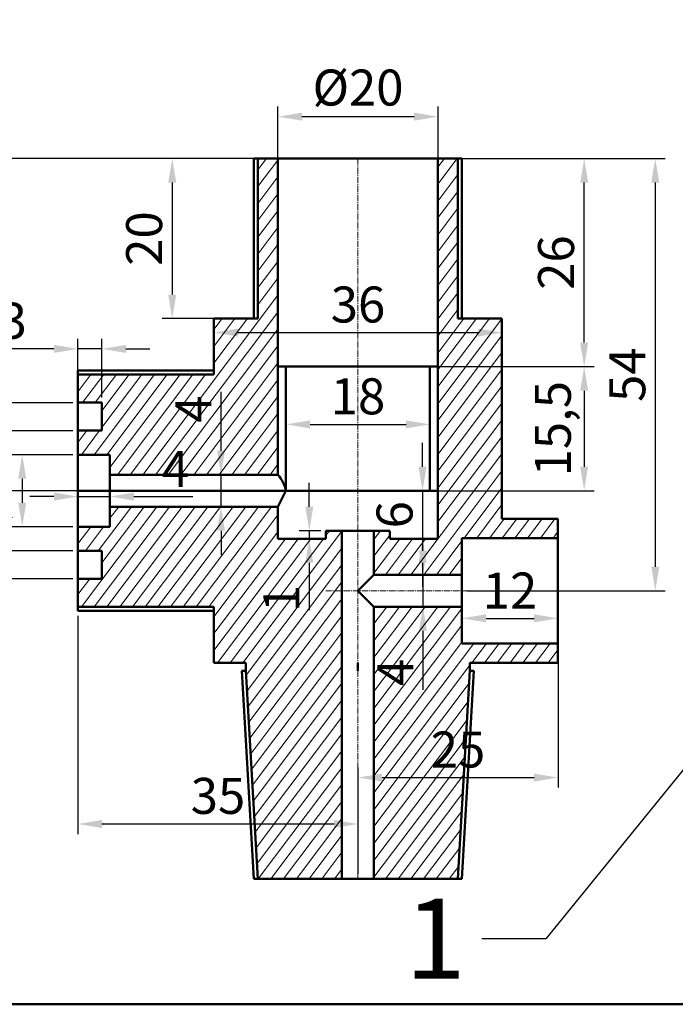
# Model space of a CAD drawing. Units: millimetres. Extents: x 418 to 773, y -46 to 294.
# Tile 2 of 7: x 483 to 565, y -46 to 77. Entities that reach past the tile are written whole.
import ezdxf
from ezdxf import colors
from ezdxf.entities.mleader import LeaderData, LeaderLine
from ezdxf.math import Vec2, Vec3

# ---------------------------------------------------------------- set-up
doc = ezdxf.new("R2010")
doc.units = ezdxf.units.MM
doc.header["$LTSCALE"] = 0.2
doc.linetypes.add('CENTER2', pattern=[28.575, 19.05, -3.175, 3.175, -3.175])
for name, color, linetype, lineweight in [('M-CNTR', 1, 'CENTER2', 18), ('M-DIMS', 2, 'Continuous', 25), ('M-HATC', 8, 'Continuous', 18), ('M-OUTL', 7, 'Continuous', 50), ('M-TEXT', 3, 'Continuous', 25), ('M-TTLB', 7, 'Continuous', 50)]:
    doc.layers.add(name, color=color, linetype=linetype, lineweight=lineweight)
doc.styles.get("Standard").update_dxf_attribs({"font": 'arial.ttf'})
doc.dimstyles.new('ISO-25', dxfattribs={"dimtxt": 4.5, "dimasz": 3, "dimexe": 1.25, "dimexo": 0.625, "dimtad": 1, "dimdec": 1, "dimtxsty": 'Standard', "dimcen": 2.5, "dimadec": 0, "dimazin": 0, "dimtfac": 1, "dimtdec": 1, "dimtmove": 0, "dimatfit": 3, "dimfxl": 1, "dimarcsym": 0})

# ---------------------------------------------------------------- blocks, each defined once
blk = doc.blocks.new('*D68')
at = {"layer": 'Defpoints', "color": 0, "ltscale": 0.2, "transparency": 16777216}
for p in [(535.05, 64.41), (515.05, 55.44), (535.05, 55.44)]:
    blk.add_point(p, dxfattribs=at)
at = {"layer": 'M-DIMS', "color": 0, "lineweight": -2, "ltscale": 0.2, "transparency": 16777216}
for p, q in [((515.05, 56.06), (515.05, 65.66)), ((535.05, 56.06), (535.05, 65.66)), ((518.05, 64.41), (532.05, 64.41))]:
    blk.add_line(p, q, dxfattribs=at)
at = {"layer": 'M-DIMS', "color": 0, "ltscale": 0.2, "transparency": 16777216}
for points in [[(518.05, 64.91), (518.05, 63.91), (515.05, 64.41)], [(532.05, 64.91), (532.05, 63.91), (535.05, 64.41)]]:
    blk.add_solid(points, dxfattribs=at)
at = {"layer": 'M-DIMS', "color": 0, "ltscale": 0.2, "transparency": 16777216, "insert": (525.05, 67.46), "char_height": 4.5, "attachment_point": 5}
blk.add_mtext('%%C20', dxfattribs=at)
blk = doc.blocks.new('*D69')
at = {"layer": 'Defpoints', "color": 0, "ltscale": 0.2, "transparency": 16777216}
for p in [(529.67, 59.18), (553.32, 59.18), (529.67, 33.18)]:
    blk.add_point(p, dxfattribs=at)
at = {"layer": 'M-DIMS', "color": 0, "lineweight": -2, "ltscale": 0.2, "transparency": 16777216}
for p, q in [((530.29, 59.18), (554.57, 59.18)), ((553.32, 36.18), (553.32, 56.18)), ((530.29, 33.18), (554.57, 33.18))]:
    blk.add_line(p, q, dxfattribs=at)
at = {"layer": 'M-DIMS', "color": 0, "ltscale": 0.2, "transparency": 16777216}
for points in [[(552.82, 56.18), (553.82, 56.18), (553.32, 59.18)], [(552.82, 36.18), (553.82, 36.18), (553.32, 33.18)]]:
    blk.add_solid(points, dxfattribs=at)
at = {"layer": 'M-DIMS', "color": 0, "ltscale": 0.2, "transparency": 16777216, "insert": (550.39, 46.18), "char_height": 4.5, "attachment_point": 5, "rotation": 90}
blk.add_mtext('26', dxfattribs=at)
blk = doc.blocks.new('*D70')
at = {"layer": 'Defpoints', "color": 0, "ltscale": 0.2, "transparency": 16777216}
for p in [(494.05, 16.95), (490.05, 15.69), (494.05, 15.68)]:
    blk.add_point(p, dxfattribs=at)
at = {"layer": 'M-DIMS', "color": 0, "lineweight": -2, "ltscale": 0.2, "transparency": 16777216}
for p, q in [((490.05, 16.31), (490.05, 18.2)), ((494.05, 16.31), (494.05, 18.2)), ((487.05, 16.95), (484.05, 16.95)), ((490.05, 16.95), (494.05, 16.95)), ((497.05, 16.95), (504.41, 16.95))]:
    blk.add_line(p, q, dxfattribs=at)
at = {"layer": 'M-DIMS', "color": 0, "ltscale": 0.2, "transparency": 16777216}
for points in [[(487.05, 17.45), (487.05, 16.45), (490.05, 16.95)], [(497.05, 17.45), (497.05, 16.45), (494.05, 16.95)]]:
    blk.add_solid(points, dxfattribs=at)
at = {"layer": 'M-DIMS', "color": 0, "ltscale": 0.2, "transparency": 16777216, "insert": (502.23, 19.83), "char_height": 4.5, "attachment_point": 5}
blk.add_mtext('4', dxfattribs=at)
blk = doc.blocks.new('*D71')
at = {"layer": 'Defpoints', "color": 0, "ltscale": 0.2, "transparency": 16777216}
for p in [(490.05, 22.18), (483.08, 13.18), (490.05, 13.18)]:
    blk.add_point(p, dxfattribs=at)
at = {"layer": 'M-DIMS', "color": 0, "lineweight": -2, "ltscale": 0.2, "transparency": 16777216}
for p, q in [((489.42, 22.18), (481.83, 22.18)), ((483.08, 19.18), (483.08, 16.18)), ((489.42, 13.18), (481.83, 13.18))]:
    blk.add_line(p, q, dxfattribs=at)
at = {"layer": 'M-DIMS', "color": 0, "ltscale": 0.2, "transparency": 16777216}
for points in [[(482.58, 19.18), (483.58, 19.18), (483.08, 22.18)], [(482.58, 16.18), (483.58, 16.18), (483.08, 13.18)]]:
    blk.add_solid(points, dxfattribs=at)
at = {"layer": 'M-DIMS', "color": 0, "ltscale": 0.2, "transparency": 16777216, "insert": (480.03, 17.68), "char_height": 4.5, "attachment_point": 5, "rotation": 90}
blk.add_mtext('%%C9', dxfattribs=at)
blk = doc.blocks.new('*D72')
at = {"layer": 'Defpoints', "color": 0, "ltscale": 0.2, "transparency": 16777216}
for p in [(490.05, 25.18), (476.38, 10.18), (490.05, 10.18)]:
    blk.add_point(p, dxfattribs=at)
at = {"layer": 'M-DIMS', "color": 0, "lineweight": -2, "ltscale": 0.2, "transparency": 16777216}
for p, q in [((489.42, 25.18), (475.13, 25.18)), ((476.38, 22.18), (476.38, 13.18)), ((489.42, 10.18), (475.13, 10.18))]:
    blk.add_line(p, q, dxfattribs=at)
at = {"layer": 'M-DIMS', "color": 0, "ltscale": 0.2, "transparency": 16777216}
for points in [[(475.88, 22.18), (476.88, 22.18), (476.38, 25.18)], [(475.88, 13.18), (476.88, 13.18), (476.38, 10.18)]]:
    blk.add_solid(points, dxfattribs=at)
at = {"layer": 'M-DIMS', "color": 0, "ltscale": 0.2, "transparency": 16777216, "insert": (473.33, 17.68), "char_height": 4.5, "attachment_point": 5, "rotation": 90}
blk.add_mtext('%%C15', dxfattribs=at)
blk = doc.blocks.new('*D73')
at = {"layer": 'Defpoints', "color": 0, "ltscale": 0.2, "transparency": 16777216}
for p in [(490.05, 28.68), (469.38, 6.68), (490.05, 6.68)]:
    blk.add_point(p, dxfattribs=at)
at = {"layer": 'M-DIMS', "color": 0, "lineweight": -2, "ltscale": 0.2, "transparency": 16777216}
for p, q in [((489.42, 28.68), (468.13, 28.68)), ((469.38, 25.68), (469.38, 9.68)), ((489.42, 6.68), (468.13, 6.68))]:
    blk.add_line(p, q, dxfattribs=at)
at = {"layer": 'M-DIMS', "color": 0, "ltscale": 0.2, "transparency": 16777216}
for points in [[(468.88, 25.68), (469.88, 25.68), (469.38, 28.68)], [(468.88, 9.68), (469.88, 9.68), (469.38, 6.68)]]:
    blk.add_solid(points, dxfattribs=at)
at = {"layer": 'M-DIMS', "color": 0, "ltscale": 0.2, "transparency": 16777216, "insert": (466.33, 17.68), "char_height": 4.5, "attachment_point": 5, "rotation": 90}
blk.add_mtext('%%C22', dxfattribs=at)
blk = doc.blocks.new('*D74')
at = {"layer": 'Defpoints', "color": 0, "ltscale": 0.2, "transparency": 16777216}
for p in [(507.93, 19.68), (510.87, 19.68), (510.87, 15.68)]:
    blk.add_point(p, dxfattribs=at)
at = {"layer": 'M-DIMS', "color": 0, "lineweight": -2, "ltscale": 0.2, "transparency": 16777216}
for p, q in [((507.93, 22.68), (507.93, 30.05)), ((510.24, 19.68), (506.68, 19.68)), ((507.93, 15.68), (507.93, 19.68)), ((510.24, 15.68), (506.68, 15.68)), ((507.93, 12.68), (507.93, 9.68))]:
    blk.add_line(p, q, dxfattribs=at)
at = {"layer": 'M-DIMS', "color": 0, "ltscale": 0.2, "transparency": 16777216}
for points in [[(507.43, 22.68), (508.43, 22.68), (507.93, 19.68)], [(507.43, 12.68), (508.43, 12.68), (507.93, 15.68)]]:
    blk.add_solid(points, dxfattribs=at)
at = {"layer": 'M-DIMS', "color": 0, "ltscale": 0.2, "transparency": 16777216, "insert": (505.05, 27.87), "char_height": 4.5, "attachment_point": 5, "rotation": 90}
blk.add_mtext('4', dxfattribs=at)
blk = doc.blocks.new('*D75')
at = {"layer": 'Defpoints', "color": 0, "ltscale": 0.2, "transparency": 16777216}
for p in [(532.4, 17.68), (532.4, 11.68), (533.12, 11.68)]:
    blk.add_point(p, dxfattribs=at)
at = {"layer": 'M-DIMS', "color": 0, "lineweight": -2, "ltscale": 0.2, "transparency": 16777216}
for p, q in [((533.12, 20.68), (533.12, 23.68)), ((533.02, 17.68), (534.37, 17.68)), ((533.12, 17.68), (533.12, 11.68)), ((533.02, 11.68), (534.37, 11.68)), ((533.12, 8.68), (533.12, 5.68))]:
    blk.add_line(p, q, dxfattribs=at)
at = {"layer": 'M-DIMS', "color": 0, "ltscale": 0.2, "transparency": 16777216}
for points in [[(532.62, 20.68), (533.62, 20.68), (533.12, 17.68)], [(532.62, 8.68), (533.62, 8.68), (533.12, 11.68)]]:
    blk.add_solid(points, dxfattribs=at)
at = {"layer": 'M-DIMS', "color": 0, "ltscale": 0.2, "transparency": 16777216, "insert": (530.2, 14.68), "char_height": 4.5, "attachment_point": 5, "rotation": 90}
blk.add_mtext('6', dxfattribs=at)
blk = doc.blocks.new('*D76')
at = {"layer": 'Defpoints', "color": 0, "ltscale": 0.2, "transparency": 16777216}
for p in [(521.05, 12.68), (518.96, 11.68), (521.05, 11.68)]:
    blk.add_point(p, dxfattribs=at)
at = {"layer": 'M-DIMS', "color": 0, "lineweight": -2, "ltscale": 0.2, "transparency": 16777216}
for p, q in [((518.96, 15.68), (518.96, 18.68)), ((520.42, 12.68), (517.71, 12.68)), ((518.96, 12.68), (518.96, 11.68)), ((520.42, 11.68), (517.71, 11.68)), ((518.96, 8.68), (518.96, 2.78))]:
    blk.add_line(p, q, dxfattribs=at)
at = {"layer": 'M-DIMS', "color": 0, "ltscale": 0.2, "transparency": 16777216}
for points in [[(518.46, 15.68), (519.46, 15.68), (518.96, 12.68)], [(518.46, 8.68), (519.46, 8.68), (518.96, 11.68)]]:
    blk.add_solid(points, dxfattribs=at)
at = {"layer": 'M-DIMS', "color": 0, "ltscale": 0.2, "transparency": 16777216, "insert": (516.07, 4.23), "char_height": 4.5, "attachment_point": 5, "rotation": 90}
blk.add_mtext('1', dxfattribs=at)
blk = doc.blocks.new('*D77')
at = {"layer": 'Defpoints', "color": 0, "ltscale": 0.2, "transparency": 16777216}
for p in [(525.05, 59.18), (501.83, 39.18), (509.8, 39.18)]:
    blk.add_point(p, dxfattribs=at)
at = {"layer": 'M-DIMS', "color": 0, "lineweight": -2, "ltscale": 0.2, "transparency": 16777216}
for p, q in [((524.42, 59.18), (500.58, 59.18)), ((501.83, 56.18), (501.83, 42.18)), ((509.17, 39.18), (500.58, 39.18))]:
    blk.add_line(p, q, dxfattribs=at)
at = {"layer": 'M-DIMS', "color": 0, "ltscale": 0.2, "transparency": 16777216}
for points in [[(501.33, 56.18), (502.33, 56.18), (501.83, 59.18)], [(501.33, 42.18), (502.33, 42.18), (501.83, 39.18)]]:
    blk.add_solid(points, dxfattribs=at)
at = {"layer": 'M-DIMS', "color": 0, "ltscale": 0.2, "transparency": 16777216, "insert": (498.9, 49.18), "char_height": 4.5, "attachment_point": 5, "rotation": 90}
blk.add_mtext('20', dxfattribs=at)
blk = doc.blocks.new('*D78')
at = {"layer": 'Defpoints', "color": 0, "ltscale": 0.2, "transparency": 16777216}
for p in [(493.05, 35.4), (490.05, 28.68), (493.05, 28.68)]:
    blk.add_point(p, dxfattribs=at)
at = {"layer": 'M-DIMS', "color": 0, "lineweight": -2, "ltscale": 0.2, "transparency": 16777216}
for p, q in [((490.05, 29.31), (490.05, 36.65)), ((493.05, 29.31), (493.05, 36.65)), ((487.05, 35.4), (479.85, 35.4)), ((493.05, 35.4), (490.05, 35.4)), ((496.05, 35.4), (499.05, 35.4))]:
    blk.add_line(p, q, dxfattribs=at)
at = {"layer": 'M-DIMS', "color": 0, "ltscale": 0.2, "transparency": 16777216}
for points in [[(487.05, 35.9), (487.05, 34.9), (490.05, 35.4)], [(496.05, 35.9), (496.05, 34.9), (493.05, 35.4)]]:
    blk.add_solid(points, dxfattribs=at)
at = {"layer": 'M-DIMS', "color": 0, "ltscale": 0.2, "transparency": 16777216, "insert": (481.95, 38.33), "char_height": 4.5, "attachment_point": 5}
blk.add_mtext('3', dxfattribs=at)
blk = doc.blocks.new('*D79')
at = {"layer": 'Defpoints', "color": 0, "ltscale": 0.2, "transparency": 16777216}
for p in [(538.05, 3.18), (550.05, 3.18), (550.05, 1.74)]:
    blk.add_point(p, dxfattribs=at)
at = {"layer": 'M-DIMS', "color": 0, "lineweight": -2, "ltscale": 0.2, "transparency": 16777216}
for p, q in [((538.05, 2.56), (538.05, 0.49)), ((550.05, 2.56), (550.05, 0.49)), ((541.05, 1.74), (547.05, 1.74))]:
    blk.add_line(p, q, dxfattribs=at)
at = {"layer": 'M-DIMS', "color": 0, "ltscale": 0.2, "transparency": 16777216}
for points in [[(541.05, 2.24), (541.05, 1.24), (538.05, 1.74)], [(547.05, 2.24), (547.05, 1.24), (550.05, 1.74)]]:
    blk.add_solid(points, dxfattribs=at)
at = {"layer": 'M-DIMS', "color": 0, "ltscale": 0.2, "transparency": 16777216, "insert": (544.05, 4.63), "char_height": 4.5, "attachment_point": 5}
blk.add_mtext('12', dxfattribs=at)
blk = doc.blocks.new('*D80')
at = {"layer": 'Defpoints', "color": 0, "ltscale": 0.2, "transparency": 16777216}
for p in [(530.7, 7.18), (530.7, 3.18), (533.17, 3.18)]:
    blk.add_point(p, dxfattribs=at)
at = {"layer": 'M-DIMS', "color": 0, "lineweight": -2, "ltscale": 0.2, "transparency": 16777216}
for p, q in [((533.17, 10.18), (533.17, 13.18)), ((531.33, 7.18), (534.42, 7.18)), ((533.17, 7.18), (533.17, 3.18)), ((531.33, 3.18), (534.42, 3.18)), ((533.17, 0.18), (533.17, -7.18))]:
    blk.add_line(p, q, dxfattribs=at)
at = {"layer": 'M-DIMS', "color": 0, "ltscale": 0.2, "transparency": 16777216}
for points in [[(532.67, 10.18), (533.67, 10.18), (533.17, 7.18)], [(532.67, 0.18), (533.67, 0.18), (533.17, 3.18)]]:
    blk.add_solid(points, dxfattribs=at)
at = {"layer": 'M-DIMS', "color": 0, "ltscale": 0.2, "transparency": 16777216, "insert": (530.29, -5), "char_height": 4.5, "attachment_point": 5, "rotation": 90}
blk.add_mtext('4', dxfattribs=at)
blk = doc.blocks.new('*D81')
at = {"layer": 'Defpoints', "color": 0, "ltscale": 0.2, "transparency": 16777216}
for p in [(529.67, 33.18), (529.67, 17.68), (553.32, 17.68)]:
    blk.add_point(p, dxfattribs=at)
at = {"layer": 'M-DIMS', "color": 0, "lineweight": -2, "ltscale": 0.2, "transparency": 16777216}
for p, q in [((530.29, 33.18), (554.57, 33.18)), ((553.32, 30.18), (553.32, 20.68)), ((530.29, 17.68), (554.57, 17.68))]:
    blk.add_line(p, q, dxfattribs=at)
at = {"layer": 'M-DIMS', "color": 0, "ltscale": 0.2, "transparency": 16777216}
for points in [[(552.82, 30.18), (553.82, 30.18), (553.32, 33.18)], [(552.82, 20.68), (553.82, 20.68), (553.32, 17.68)]]:
    blk.add_solid(points, dxfattribs=at)
at = {"layer": 'M-DIMS', "color": 0, "ltscale": 0.2, "transparency": 16777216, "insert": (549.99, 25.43), "char_height": 4.5, "attachment_point": 5, "rotation": 90}
blk.add_mtext('15,5', dxfattribs=at)
blk = doc.blocks.new('*D82')
at = {"layer": 'Defpoints', "color": 0, "ltscale": 0.2, "transparency": 16777216}
for p in [(516.05, 26.43), (534.05, 26.43), (534.05, 25.97)]:
    blk.add_point(p, dxfattribs=at)
at = {"layer": 'M-DIMS', "color": 0, "lineweight": -2, "ltscale": 0.2, "transparency": 16777216}
for p, q in [((519.05, 25.97), (531.05, 25.97)), ((516.05, 25.81), (516.05, 24.72)), ((534.05, 25.81), (534.05, 24.72))]:
    blk.add_line(p, q, dxfattribs=at)
at = {"layer": 'M-DIMS', "color": 0, "ltscale": 0.2, "transparency": 16777216}
for points in [[(519.05, 26.47), (519.05, 25.47), (516.05, 25.97)], [(531.05, 26.47), (531.05, 25.47), (534.05, 25.97)]]:
    blk.add_solid(points, dxfattribs=at)
at = {"layer": 'M-DIMS', "color": 0, "ltscale": 0.2, "transparency": 16777216, "insert": (525.05, 28.89), "char_height": 4.5, "attachment_point": 5}
blk.add_mtext('18', dxfattribs=at)
blk = doc.blocks.new('*D83')
at = {"layer": 'Defpoints', "color": 0, "ltscale": 0.2, "transparency": 16777216}
for p in [(543.05, 37.44), (507.05, 35.93), (543.05, 35.93)]:
    blk.add_point(p, dxfattribs=at)
at = {"layer": 'M-DIMS', "color": 0, "lineweight": -2, "ltscale": 0.2, "transparency": 16777216}
for p, q in [((507.05, 36.56), (507.05, 38.69)), ((543.05, 36.56), (543.05, 38.69)), ((510.05, 37.44), (540.05, 37.44))]:
    blk.add_line(p, q, dxfattribs=at)
at = {"layer": 'M-DIMS', "color": 0, "ltscale": 0.2, "transparency": 16777216}
for points in [[(510.05, 37.94), (510.05, 36.94), (507.05, 37.44)], [(540.05, 37.94), (540.05, 36.94), (543.05, 37.44)]]:
    blk.add_solid(points, dxfattribs=at)
at = {"layer": 'M-DIMS', "color": 0, "ltscale": 0.2, "transparency": 16777216, "insert": (525.05, 40.36), "char_height": 4.5, "attachment_point": 5}
blk.add_mtext('36', dxfattribs=at)
blk = doc.blocks.new('*D84')
at = {"layer": 'Defpoints', "color": 0, "ltscale": 0.2, "transparency": 16777216}
for p in [(550.05, 5.18), (550.05, -18.15), (525.05, -30.82)]:
    blk.add_point(p, dxfattribs=at)
at = {"layer": 'M-DIMS', "color": 0, "lineweight": -2, "ltscale": 0.2, "transparency": 16777216}
for p, q in [((550.05, 4.56), (550.05, -19.4)), ((525.05, -30.19), (525.05, -16.9)), ((528.05, -18.15), (547.05, -18.15))]:
    blk.add_line(p, q, dxfattribs=at)
at = {"layer": 'M-DIMS', "color": 0, "ltscale": 0.2, "transparency": 16777216}
for points in [[(528.05, -17.65), (528.05, -18.65), (525.05, -18.15)], [(547.05, -17.65), (547.05, -18.65), (550.05, -18.15)]]:
    blk.add_solid(points, dxfattribs=at)
at = {"layer": 'M-DIMS', "color": 0, "ltscale": 0.2, "transparency": 16777216, "insert": (537.55, -15.23), "char_height": 4.5, "attachment_point": 5}
blk.add_mtext('25', dxfattribs=at)
blk = doc.blocks.new('*D85')
at = {"layer": 'Defpoints', "color": 0, "ltscale": 0.2, "transparency": 16777216}
for p in [(490.05, 2.68), (490.05, -23.95), (525.05, -30.82)]:
    blk.add_point(p, dxfattribs=at)
at = {"layer": 'M-DIMS', "color": 0, "lineweight": -2, "ltscale": 0.2, "transparency": 16777216}
for p, q in [((490.05, 2.06), (490.05, -25.2)), ((525.05, -30.19), (525.05, -22.7)), ((522.05, -23.95), (493.05, -23.95))]:
    blk.add_line(p, q, dxfattribs=at)
at = {"layer": 'M-DIMS', "color": 0, "ltscale": 0.2, "transparency": 16777216}
for points in [[(493.05, -23.45), (493.05, -24.45), (490.05, -23.95)], [(522.05, -23.45), (522.05, -24.45), (525.05, -23.95)]]:
    blk.add_solid(points, dxfattribs=at)
at = {"layer": 'M-DIMS', "color": 0, "ltscale": 0.2, "transparency": 16777216, "insert": (507.55, -21.02), "char_height": 4.5, "attachment_point": 5}
blk.add_mtext('35', dxfattribs=at)
blk = doc.blocks.new('*D86')
at = {"layer": 'Defpoints', "color": 0, "ltscale": 0.2, "transparency": 16777216}
for p in [(525.05, 59.18), (457.05, 17.68), (525.05, 17.68)]:
    blk.add_point(p, dxfattribs=at)
at = {"layer": 'M-DIMS', "color": 0, "lineweight": -2, "ltscale": 0.2, "transparency": 16777216}
for p, q in [((524.42, 59.18), (455.8, 59.18)), ((457.05, 56.18), (457.05, 20.68)), ((524.42, 17.68), (455.8, 17.68))]:
    blk.add_line(p, q, dxfattribs=at)
at = {"layer": 'M-DIMS', "color": 0, "ltscale": 0.2, "transparency": 16777216}
for points in [[(456.55, 56.18), (457.55, 56.18), (457.05, 59.18)], [(456.55, 20.68), (457.55, 20.68), (457.05, 17.68)]]:
    blk.add_solid(points, dxfattribs=at)
at = {"layer": 'M-DIMS', "color": 0, "ltscale": 0.2, "transparency": 16777216, "insert": (453.72, 38.43), "char_height": 4.5, "attachment_point": 5, "rotation": 90}
blk.add_mtext('41,5', dxfattribs=at)
blk = doc.blocks.new('*D89')
at = {"layer": 'Defpoints', "color": 0, "ltscale": 0.2, "transparency": 16777216}
for p in [(538.05, 59.18), (538.05, 5.18), (562.21, 5.18)]:
    blk.add_point(p, dxfattribs=at)
at = {"layer": 'M-DIMS', "color": 0, "lineweight": -2, "ltscale": 0.2, "transparency": 16777216}
for p, q in [((538.67, 59.18), (563.46, 59.18)), ((562.21, 56.18), (562.21, 8.18)), ((538.67, 5.18), (563.46, 5.18))]:
    blk.add_line(p, q, dxfattribs=at)
at = {"layer": 'M-DIMS', "color": 0, "ltscale": 0.2, "transparency": 16777216}
for points in [[(561.71, 56.18), (562.71, 56.18), (562.21, 59.18)], [(561.71, 8.18), (562.71, 8.18), (562.21, 5.18)]]:
    blk.add_solid(points, dxfattribs=at)
at = {"layer": 'M-DIMS', "color": 0, "ltscale": 0.2, "transparency": 16777216, "insert": (559.29, 32.18), "char_height": 4.5, "attachment_point": 5, "rotation": 90}
blk.add_mtext('54', dxfattribs=at)

msp = doc.modelspace()

# ---------------------------------------------------------------- hatches: boundary and pattern name
at = {"layer": 'M-HATC', "ltscale": 0.2}
h = msp.add_hatch(dxfattribs=at)
h.set_pattern_fill('ANSI31', color=256, scale=0.4, angle=8)
h.set_pattern_definition([(53, (-436.446, -169.6486), (-1.0142671, 0.764305), [])])
h.paths.add_polyline_path([(527.0464, -30.8151), (537.5456, -30.8151), (539.0472, -4.7863), (539.0472, -3.8151), (550.0464, -3.8151), (550.0464, -1.3951), (538.0464, -1.3951), (538.0464, 3.1849), (527.0464, 3.1849)])
h.paths.add_polyline_path([(538.0464, 11.7649), (550.0464, 11.7649), (550.0464, 14.1849), (543.0464, 14.1849), (543.0464, 39.1849), (537.5464, 39.1849), (537.5464, 59.1849), (535.0464, 59.1849), (535.0464, 33.1849), (535.0464, 17.6849), (535.0464, 11.6849), (529.0464, 11.6849), (529.0464, 12.6849), (527.0464, 12.6849), (527.0464, 7.1849), (538.0464, 7.1849)])
h.paths.add_polyline_path([(515.0464, 33.1849), (515.0464, 59.1849), (512.5464, 59.1849), (512.5464, 39.1849), (507.0464, 39.1849), (507.0464, 32.1849), (490.0464, 32.1849), (490.0464, 28.6849), (493.0464, 28.6849), (493.0464, 25.1849), (490.0464, 25.1849), (490.0464, 22.1849), (494.0464, 22.1849), (494.0464, 19.6849), (515.0464, 19.6849)])
h.paths.add_polyline_path([(507.0464, 3.1849), (507.0464, -3.8151), (511.0464, -3.8151), (511.0464, -4.8007), (512.5472, -30.8151), (523.0464, -30.8151), (523.0464, 12.6849), (521.0464, 12.6849), (521.0464, 11.6849), (515.0464, 11.6849), (515.0464, 15.6849), (494.0464, 15.6849), (494.0464, 13.1849), (490.0464, 13.1849), (490.0464, 10.1849), (493.0464, 10.1849), (493.0464, 6.6849), (490.0464, 6.6849), (490.0464, 3.1849)])

# ---------------------------------------------------------------- linework, layer by layer
at = {"layer": 'M-CNTR', "ltscale": 0.2}
for p, q in [((525.0464, 59.1849), (525.0464, -30.8151)), ((551.442, 5.1849), (521.0112, 5.1849))]:
    msp.add_line(p, q, dxfattribs=at)
at = {"layer": 'M-OUTL', "ltscale": 0.2}
for p, q in [((515.0464, 59.1849), (512.0464, 59.1849)), ((512.0464, 59.1849), (512.0464, 39.1849)), ((512.5464, 59.1849), (512.5464, 39.1849)), ((515.0464, 59.1849), (535.0464, 59.1849)), ((515.0464, 33.1849), (515.0464, 59.1849)), ((535.0464, 59.1849), (535.0464, 33.1849)), ((535.0464, 59.1849), (538.0464, 59.1849)), ((537.5464, 59.1849), (537.5464, 39.1849)), ((538.0464, 59.1849), (538.0464, 39.1849)), ((512.5464, 39.1849), (507.0464, 39.1849)), ((507.0464, 39.1849), (507.0464, 32.6849)), ((507.0464, 32.1849), (507.0464, 39.1849)), ((537.5464, 39.1849), (543.0464, 39.1849)), ((543.0464, 39.1849), (543.0464, 14.1849)), ((490.0464, 17.6849), (490.0464, 32.6849)), ((490.0464, 17.6849), (490.0464, 32.6849)), ((490.0464, 32.6849), (507.0464, 32.6849)), ((490.0464, 32.1849), (507.0464, 32.1849)), ((535.0464, 33.1849), (515.0464, 33.1849)), ((515.0464, 33.1849), (515.0464, 19.6849)), ((516.0464, 17.6849), (516.0464, 33.1849)), ((534.0464, 33.1849), (534.0464, 17.6849)), ((535.0464, 33.1849), (535.0464, 17.6849)), ((490.0464, 28.6849), (493.0464, 28.6849)), ((493.0464, 28.6849), (493.0464, 25.1849)), ((493.0464, 25.1849), (490.0464, 25.1849)), ((490.0464, 22.1849), (494.0464, 22.1849)), ((494.0464, 22.1849), (494.0464, 13.1849)), ((494.0464, 19.6849), (515.0464, 19.6849)), ((490.0464, 17.6849), (535.0464, 17.6849)), ((490.0464, 17.6849), (490.0464, 2.6849)), ((515.0464, 15.6849), (516.0464, 17.6849)), ((535.0464, 17.6849), (535.0464, 11.6849)), ((494.0464, 15.6849), (515.0464, 15.6849)), ((515.0464, 15.6849), (515.0464, 11.6849)), ((550.0464, 14.1849), (543.0464, 14.1849)), ((550.0464, 5.1849), (550.0464, 14.1849)), ((494.0464, 13.1849), (490.0464, 13.1849)), ((521.0464, 12.6849), (525.0464, 12.6849)), ((521.0464, 12.6849), (521.0464, 11.6849)), ((523.0464, 12.6849), (523.0464, -30.8151)), ((529.0464, 12.6849), (525.0464, 12.6849)), ((527.0464, 12.6849), (527.0464, 7.1849)), ((529.0464, 11.6849), (529.0464, 12.6849)), ((515.0464, 11.6849), (521.0464, 11.6849)), ((535.0464, 11.6849), (529.0464, 11.6849)), ((550.0464, 11.7649), (538.0464, 11.7649)), ((538.0464, 11.7649), (538.0464, -1.3951)), ((493.0464, 10.1849), (490.0464, 10.1849)), ((493.0464, 6.6849), (493.0464, 10.1849)), ((490.0464, 6.6849), (493.0464, 6.6849)), ((525.0464, 5.1849), (527.0464, 7.1849)), ((538.0464, 7.1849), (527.0464, 7.1849)), ((525.0464, 5.1849), (527.0464, 3.1849)), ((550.0464, 5.1849), (550.0464, -3.8151)), ((490.0464, 3.1849), (507.0464, 3.1849)), ((490.0464, 2.6849), (507.0464, 2.6849)), ((507.0464, 3.1849), (507.0464, -3.8151)), ((538.0464, 3.1849), (527.0464, 3.1849)), ((527.0464, 3.1849), (527.0464, -30.8151)), ((538.0464, -1.3951), (550.0464, -1.3951)), ((511.0464, -3.8151), (507.0464, -3.8151)), ((510.5464, -4.8151), (511.0472, -4.8151)), ((510.5464, -4.8151), (512.0464, -30.8151)), ((511.0456, -4.7863), (512.5456, -30.7863)), ((511.0464, -4.8151), (511.0464, -3.8151)), ((525.0464, -3.8151), (525.0464, -4.8151)), ((539.0472, -4.7863), (537.5472, -30.7863)), ((538.0464, -30.8151), (539.5464, -4.8151)), ((539.0456, -4.8151), (539.5464, -4.8151)), ((550.0464, -3.8151), (539.0472, -3.8151)), ((539.0472, -4.7863), (539.0472, -3.8151)), ((512.0464, -30.8151), (538.0464, -30.8151)), ((525.0464, -30.8151), (523.0464, -30.8151)), ((525.0464, -30.8151), (538.0464, -30.8151))]:
    msp.add_line(p, q, dxfattribs=at)
msp.add_arc((511.3262, 16.5748), 4.849, 13.234399, 39.895704, dxfattribs=at)
at = {"layer": 'M-TTLB', "ltscale": 0.2}
msp.add_lwpolyline([(417.9371, 294.4119), (773.2687, 294.4119), (773.2687, -46.4726), (417.9371, -46.4726)], close=True, dxfattribs=at)

# ---------------------------------------------------------------- dimensions: what is measured, and where the dimension line sits
at = {"layer": 'M-DIMS', "ltscale": 0.2}
dim = msp.add_linear_dim(base=(535.0464, 64.4103), p1=(515.0464, 55.4365), p2=(535.0464, 55.4365), text='%%C<>', dimstyle='ISO-25', override={"dimclrd": 0, "dimclre": 0, "dimclrt": 0}, dxfattribs=at)
dim.commit()
dim.dimension.update_dxf_attribs({"geometry": '*D68', "text_midpoint": (525.0464, 67.4587)})
for base, p1, p2, picture, middle in [((457.0454, 17.6849), (525.0464, 59.1849), (525.0464, 17.6849), '*D86', (453.7161, 38.4349)), ((501.8268, 39.1849), (525.0464, 59.1849), (509.7964, 39.1849), '*D77', (498.9042, 49.1849)), ((553.3174, 59.1849), (529.6673, 33.1849), (529.6673, 59.1849), '*D69', (550.3948, 46.1849)), ((562.2053, 5.1849), (538.0464, 59.1849), (538.0464, 5.1849), '*D89', (559.2919, 32.1849)), ((553.3174, 17.6849), (529.6673, 33.1849), (529.6673, 17.6849), '*D81', (549.9881, 25.4349)), ((507.9273, 19.6849), (510.8656, 15.6849), (510.8656, 19.6849), '*D74', (505.0523, 27.8662)), ((533.1226, 11.6849), (532.3989, 17.6849), (532.3989, 11.6849), '*D75', (530.2, 14.6849)), ((518.9577, 11.6849), (521.0464, 12.6849), (521.0464, 11.6849), '*D76', (516.0735, 4.2311)), ((533.1658, 3.1849), (530.7015, 7.1849), (530.7015, 3.1849), '*D80', (530.2908, -4.9964))]:
    dim = msp.add_linear_dim(base=base, p1=p1, p2=p2, angle=90, dimstyle='ISO-25', override={"dimclrd": 0, "dimclre": 0, "dimclrt": 0}, dxfattribs=at)
    dim.commit()
    dim.dimension.update_dxf_attribs({"geometry": picture, "text_midpoint": middle})
for base, p1, p2, picture, middle in [((543.0464, 37.436), (507.0464, 35.9349), (543.0464, 35.9349), '*D83', (525.0464, 40.3601)), ((534.0464, 25.9679), (516.0464, 26.4349), (534.0464, 26.4349), '*D82', (525.0464, 28.8905)), ((550.0464, 1.742), (538.0464, 3.1849), (550.0464, 3.1849), '*D79', (544.0464, 4.6262)), ((550.0464, -18.1516), (525.0464, -30.8151), (550.0464, 5.1849), '*D84', (537.5464, -15.229)), ((490.0464, -23.9483), (525.0464, -30.8151), (490.0464, 2.6849), '*D85', (507.5464, -21.0242))]:
    dim = msp.add_linear_dim(base=base, p1=p1, p2=p2, dimstyle='ISO-25', override={"dimclrd": 0, "dimclre": 0, "dimclrt": 0}, dxfattribs=at)
    dim.commit()
    dim.dimension.update_dxf_attribs({"geometry": picture, "text_midpoint": middle})
for base, p1, p2, picture, middle in [((493.0464, 35.4018), (490.0464, 28.6849), (493.0464, 28.6849), '*D78', (481.948, 35.4018)), ((494.0464, 16.9501), (490.0464, 15.6899), (494.0464, 15.6849), '*D70', (502.2277, 16.9501))]:
    dim = msp.add_linear_dim(base=base, p1=p1, p2=p2, dimstyle='ISO-25', override={"dimclrd": 0, "dimclre": 0, "dimclrt": 0}, dxfattribs=at)
    dim.commit()
    dim.dimension.update_dxf_attribs({"geometry": picture, "text_midpoint": middle, "dimtype": 160})
for base, p1, p2, picture, middle in [((469.3802, 6.6849), (490.0464, 28.6849), (490.0464, 6.6849), '*D73', (466.3318, 17.6849)), ((476.377, 10.1849), (490.0464, 25.1849), (490.0464, 10.1849), '*D72', (473.3286, 17.6849))]:
    dim = msp.add_linear_dim(base=base, p1=p1, p2=p2, angle=90, text='%%C<>', dimstyle='ISO-25', override={"dimclrd": 0, "dimclre": 0, "dimclrt": 0}, dxfattribs=at)
    dim.commit()
    dim.dimension.update_dxf_attribs({"geometry": picture, "text_midpoint": middle})
dim = msp.add_linear_dim(base=(483.0819, 13.1849), p1=(490.0464, 22.1849), p2=(490.0464, 13.1849), angle=90, text='%%C<>', dimstyle='ISO-25', override={"dimclrd": 0, "dimclre": 0, "dimclrt": 0}, dxfattribs=at)
dim.commit()
dim.dimension.update_dxf_attribs({"geometry": '*D71', "text_midpoint": (483.0819, 17.6849), "dimtype": 160})

# ---------------------------------------------------------------- leaders
at = {"layer": 'M-TEXT', "ltscale": 0.2}
ml = msp.add_multileader_mtext('Standard', dxfattribs=at)
ml.set_content('1', color=256)
ml.set_leader_properties()
ml.build(insert=Vec2(0, 0))
ctx = ml.context
ctx.base_point, ctx.char_height, ctx.plane_origin = Vec3(532.8405, -38.2871), 10, Vec3(571.5171, -9.9875)
ctx.text_align_type = 2
notes = []
notes.append((ctx, [(0, (1, 1, 0), (548.5239, -38.2871), (-1, 0), 8, [(0, [(571.5171, -9.9875)], 0, [])])]))
ctx.mtext.insert, ctx.mtext.alignment, ctx.mtext.flow_direction = Vec3(538.5239, -33.2871), 3, 5
for ctx, leaders in notes:
    for number, flags, end, landing, length, lines in leaders:
        leader = LeaderData()
        leader.index, (leader.has_last_leader_line, leader.has_dogleg_vector, leader.attachment_direction) = number, flags
        leader.last_leader_point, leader.dogleg_vector, leader.dogleg_length = Vec3(end), Vec3(landing), length
        for number, points, colour, breaks in lines:
            line = LeaderLine()
            line.index, line.vertices, line.color, line.breaks = number, Vec3.list(points), colors.encode_raw_color(colour), breaks
            leader.lines.append(line)
        ctx.leaders.append(leader)

doc.saveas('drawing.dxf')
